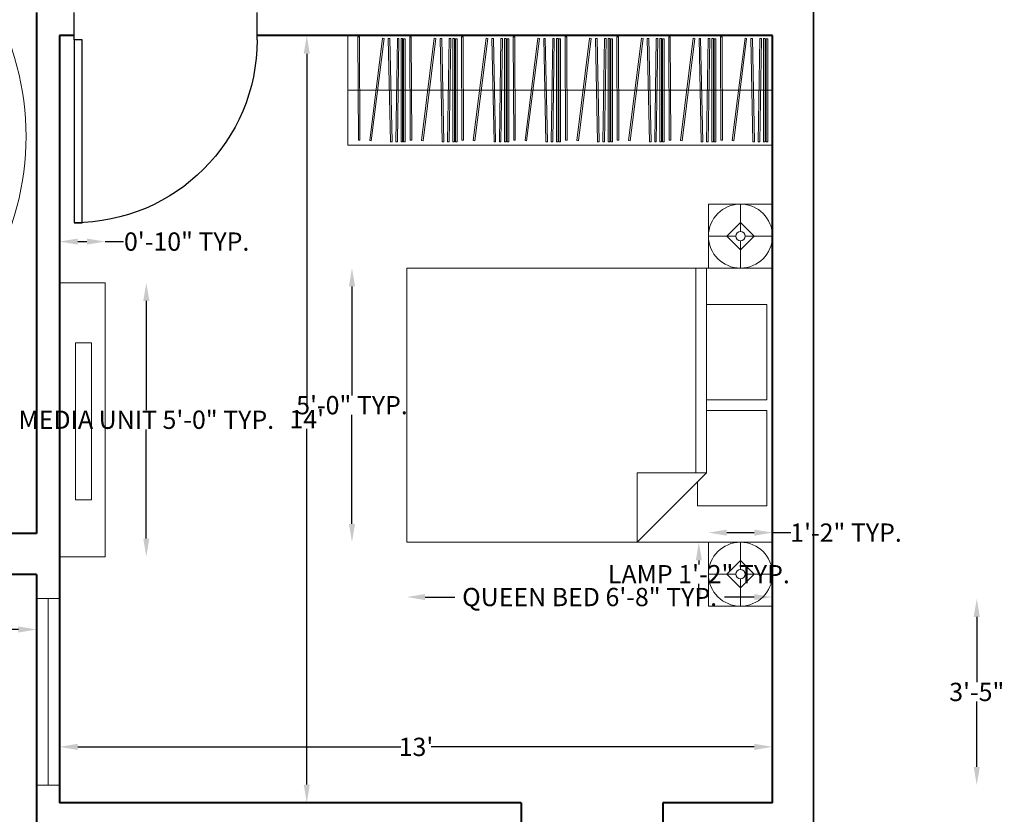
# Model space of a CAD drawing. Units: inches. Extents: x -46 to 447, y -42 to 702.
# Tile 3 of 7: x 222 to 438, y 148 to 322. Entities that reach past the tile are written whole.
import ezdxf

# ---------------------------------------------------------------- set-up
doc = ezdxf.new("R2010")
doc.units = ezdxf.units.IN
doc.header["$PDMODE"] = 3
for name, color, linetype, lineweight in [('A-ANNO-DIMS', 2, 'Continuous', 13), ('A-DOOR', 3, 'Continuous', 25), ('A-FLOR-CASE', 32, 'Continuous', 18), ('A-FURN', 8, 'Continuous', 18), ('A-GLAZ', 4, 'Continuous', 18), ('A-WALL', 7, 'Continuous', 40), ('L-WALL', 7, 'Continuous', 35)]:
    doc.layers.add(name, color=color, linetype=linetype, lineweight=lineweight)
doc.styles.get("Standard").update_dxf_attribs({"font": 'arial.ttf'})
doc.dimstyles.get("Standard").update_dxf_attribs({"dimtxt": 4, "dimasz": 4, "dimexe": 0.18, "dimexo": 0.0625, "dimgap": 0.09, "dimtad": 0, "dimtih": 1, "dimtoh": 1, "dimdec": 0, "dimzin": 0, "dimdsep": 46, "dimlunit": 3, "dimtxsty": 'Standard', "dimcen": 0.09, "dimse1": 1, "dimse2": 1, "dimadec": 0, "dimazin": 0, "dimtfac": 1, "dimtdec": 0, "dimtofl": 0, "dimtmove": 0, "dimatfit": 3, "dimfxl": 1, "dimtolj": 1, "dimtzin": 0, "dimarcsym": 0})

# ---------------------------------------------------------------- blocks, each defined once
blk = doc.blocks.new('*U2')
for p, q in [((0, 0), (0, -6)), ((40, 0), (40, -6))]:
    blk.add_line(p, q)
blk.add_lwpolyline([(0, 0), (0, 40), (1.75, 40), (1.75, 0)], close=True)
blk.add_arc((0, 0), 40, 0, 90)
blk = doc.blocks.new('Sofa - Roundback Loveseat 5 ft.')
for p, q in [((0, -32.44198), (0, -5.99998)), ((-24, -33.99998), (-24, -11.46958)), ((24.00004, -33.99998), (24.00004, -11.46958)), ((-23.9998, -13.38178), (23.99986, -13.38178)), ((-24, -32.44198), (24.00004, -32.44198))]:
    blk.add_line(p, q)
for points in [[(-24, -33.99998), (-30, -33.99998), (-30, -7.99998)], [(30.00004, -7.99998), (30.00004, -33.99998), (24.00004, -33.99998)]]:
    blk.add_lwpolyline(points)
for centre, radius, start, end in [((0, -60.24998), 60.24998, 60.13715, 119.8628), ((0, -61.38438), 55.38444, 64.32083, 115.6792)]:
    blk.add_arc(centre, radius, start, end)
blk = doc.blocks.new('Bed - Queen')
for p, q in [((0, -80.00003), (0, 0)), ((0, 0), (59.99999, 0)), ((59.99999, 0), (59.99999, -80.00003)), ((7.99999, -1.2), (28.79998, -1.2)), ((7.99999, -14.4), (7.99999, -1.2)), ((28.79998, -1.2), (28.79998, -14.4)), ((31.19999, -1.2), (51.99999, -1.2)), ((31.19999, -14.4), (31.19999, -1.2)), ((51.99999, -1.2), (51.99999, -16.4)), ((0, -14.4), (44.8, -14.4)), ((59.99999, -29.6), (44.8, -14.4)), ((44.8, -14.4), (44.8, -29.6)), ((44.8, -16.8), (0, -16.8)), ((51.99999, -16.4), (46.79936, -16.4)), ((44.8, -29.6), (59.99999, -29.6)), ((59.99999, -80.00003), (0, -80.00003))]:
    blk.add_line(p, q)
blk = doc.blocks.new('Lamp - Table')
for p, q in [((0, 7), (0, 1)), ((0, 3), (-3, 0)), ((3, 0), (0, 3)), ((-1, 0), (-7, 0)), ((-3, 0), (0, -3)), ((0, -3), (3, 0)), ((1, 0), (7, 0)), ((0, -1), (0, -7))]:
    blk.add_line(p, q)
for radius in [7, 1]:
    blk.add_circle((0, 0), radius)
blk = doc.blocks.new('*D52')
at = {"layer": 'A-ANNO-DIMS', "color": 0, "lineweight": -2, "transparency": 16777216}
for p, q in [((13, 188.95), (110.73, 188.95)), ((222, 188.95), (124.27, 188.95))]:
    blk.add_line(p, q, dxfattribs=at)
at = {"layer": 'A-ANNO-DIMS', "color": 0, "transparency": 16777216}
for points in [[(13, 189.62), (13, 188.29), (9, 188.95)], [(222, 189.62), (222, 188.29), (226, 188.95)]]:
    blk.add_solid(points, dxfattribs=at)
at = {"layer": 'Defpoints', "color": 0, "transparency": 16777216}
for p in [(226, 188.95), (9, 180.86), (226, 180.86)]:
    blk.add_point(p, dxfattribs=at)
at = {"layer": 'A-ANNO-DIMS', "color": 0, "transparency": 16777216, "insert": (117.5, 188.95), "char_height": 4, "attachment_point": 5}
blk.add_mtext('\\A1;18\'-1"', dxfattribs=at)
blk = doc.blocks.new('*D59')
at = {"layer": 'A-ANNO-DIMS', "color": 0, "lineweight": -2, "transparency": 16777216}
for p, q in [((285.11, 315), (285.11, 237.1)), ((285.11, 155), (285.11, 232.9))]:
    blk.add_line(p, q, dxfattribs=at)
at = {"layer": 'A-ANNO-DIMS', "color": 0, "transparency": 16777216}
for points in [[(284.44, 315), (285.78, 315), (285.11, 319)], [(284.44, 155), (285.78, 155), (285.11, 151)]]:
    blk.add_solid(points, dxfattribs=at)
at = {"layer": 'Defpoints', "color": 0, "transparency": 16777216}
for p in [(285.11, 319), (387, 319), (387, 151)]:
    blk.add_point(p, dxfattribs=at)
at = {"layer": 'A-ANNO-DIMS', "color": 0, "transparency": 16777216, "insert": (285.11, 235), "char_height": 4, "attachment_point": 5}
blk.add_mtext("\\A1;14'", dxfattribs=at)
blk = doc.blocks.new('*D60')
at = {"layer": 'A-ANNO-DIMS', "color": 0, "lineweight": -2, "transparency": 16777216}
for p, q in [((235, 163.26), (305.7, 163.26)), ((383, 163.26), (312.3, 163.26))]:
    blk.add_line(p, q, dxfattribs=at)
at = {"layer": 'A-ANNO-DIMS', "color": 0, "transparency": 16777216}
for points in [[(235, 163.93), (235, 162.59), (231, 163.26)], [(383, 163.93), (383, 162.59), (387, 163.26)]]:
    blk.add_solid(points, dxfattribs=at)
at = {"layer": 'Defpoints', "color": 0, "transparency": 16777216}
for p in [(387, 163.26), (231, 151), (387, 151)]:
    blk.add_point(p, dxfattribs=at)
at = {"layer": 'A-ANNO-DIMS', "color": 0, "transparency": 16777216, "insert": (309, 163.26), "char_height": 4, "attachment_point": 5}
blk.add_mtext("\\A1;13'", dxfattribs=at)
blk = doc.blocks.new('WARDROBE-93X24')
for p, q in [((12, -92.9), (12, 0)), ((24, 0), (24, -92.9)), ((24, -92.9), (0, -92.9))]:
    blk.add_line(p, q)
for points in [[(0.7, -1.6), (23.3, -1.6), (23.3, -1.95), (0.7, -1.95)], [(0.72, -1.03), (23.33, -1.03), (23.33, -1.38), (0.72, -1.38)], [(23.3, -3.1), (0.7, -2.75), (0.7, -2.4), (23.3, -2.75)], [(23.3, -4.26), (0.7, -4.73), (0.7, -4.38), (23.3, -3.91)], [(23.09, -8.46), (0.66, -5.66), (0.61, -6), (23.04, -8.81)], [(22.92, -11.29), (0.31, -11.38), (0.31, -11.03), (22.91, -10.94)], [(0.72, -12.37), (23.33, -12.37), (23.33, -12.72), (0.72, -12.72)], [(0.7, -12.93), (23.3, -12.93), (23.3, -13.28), (0.7, -13.28)], [(23.3, -14.43), (0.7, -14.08), (0.7, -13.73), (23.3, -14.08)], [(23.09, -19.79), (0.66, -16.99), (0.61, -17.34), (23.04, -20.14)], [(23.3, -15.59), (0.7, -16.06), (0.7, -15.71), (23.3, -15.24)], [(22.92, -22.62), (0.31, -22.71), (0.31, -22.36), (22.91, -22.27)], [(0.72, -23.7), (23.33, -23.7), (23.33, -24.05), (0.72, -24.05)], [(0.7, -24.26), (23.3, -24.26), (23.3, -24.61), (0.7, -24.61)], [(23.3, -25.77), (0.7, -25.41), (0.7, -25.06), (23.3, -25.41)], [(23.3, -26.93), (0.7, -27.39), (0.7, -27.04), (23.3, -26.57)], [(23.09, -31.12), (0.66, -28.32), (0.61, -28.67), (23.04, -31.47)], [(22.92, -33.95), (0.31, -34.04), (0.31, -33.69), (22.91, -33.6)], [(0.7, -35.59), (23.3, -35.59), (23.3, -35.94), (0.7, -35.94)], [(23.3, -37.1), (0.7, -36.75), (0.7, -36.39), (23.3, -36.75)], [(0.72, -35.03), (23.33, -35.03), (23.33, -35.38), (0.72, -35.38)], [(23.3, -38.26), (0.7, -38.72), (0.7, -38.37), (23.3, -37.91)], [(23.09, -42.45), (0.66, -39.65), (0.61, -40), (23.04, -42.8)], [(22.92, -45.28), (0.31, -45.37), (0.31, -45.02), (22.91, -44.93)], [(0.7, -46.92), (23.3, -46.92), (23.3, -47.27), (0.7, -47.27)], [(0.72, -46.36), (23.33, -46.36), (23.33, -46.71), (0.72, -46.71)], [(23.3, -48.43), (0.7, -48.08), (0.7, -47.73), (23.3, -48.08)], [(23.3, -49.59), (0.7, -50.05), (0.7, -49.7), (23.3, -49.24)], [(23.09, -53.79), (0.66, -50.98), (0.61, -51.33), (23.04, -54.13)], [(22.92, -56.61), (0.31, -56.7), (0.31, -56.35), (22.91, -56.26)], [(0.72, -57.69), (23.33, -57.69), (23.33, -58.04), (0.72, -58.04)], [(0.7, -58.25), (23.3, -58.25), (23.3, -58.6), (0.7, -58.6)], [(23.3, -59.76), (0.7, -59.41), (0.7, -59.06), (23.3, -59.41)], [(23.09, -65.12), (0.66, -62.31), (0.61, -62.66), (23.04, -65.47)], [(23.3, -60.92), (0.7, -61.39), (0.7, -61.04), (23.3, -60.57)], [(22.92, -67.95), (0.31, -68.04), (0.31, -67.68), (22.91, -67.59)], [(0.7, -69.59), (23.3, -69.59), (23.3, -69.94), (0.7, -69.94)], [(23.3, -71.09), (0.7, -70.74), (0.7, -70.39), (23.3, -70.74)], [(0.72, -69.02), (23.33, -69.02), (23.33, -69.37), (0.72, -69.37)], [(23.3, -72.25), (0.7, -72.72), (0.7, -72.37), (23.3, -71.9)], [(23.09, -76.45), (0.66, -73.64), (0.61, -73.99), (23.04, -76.8)], [(22.92, -79.28), (0.31, -79.37), (0.31, -79.02), (22.91, -78.93)], [(0.7, -80.92), (23.3, -80.92), (23.3, -81.27), (0.7, -81.27)], [(23.3, -82.42), (0.7, -82.07), (0.7, -81.72), (23.3, -82.07)], [(0.72, -80.35), (23.33, -80.35), (23.33, -80.71), (0.72, -80.71)], [(23.3, -83.58), (0.7, -84.05), (0.7, -83.7), (23.3, -83.23)], [(23.09, -87.78), (0.66, -84.98), (0.61, -85.32), (23.04, -88.13)], [(22.92, -90.61), (0.31, -90.7), (0.31, -90.35), (22.91, -90.26)]]:
    blk.add_lwpolyline(points, close=True)
blk = doc.blocks.new('MEDIA-CONSOLE-60')
for points in [[(60, 0), (0, 0), (0, 10), (60, 10)], [(13.13, 6.99), (47.53, 6.99), (47.53, 3.54), (13.13, 3.54)]]:
    blk.add_lwpolyline(points, close=True)
blk = doc.blocks.new('NIGHTSTAND-14')
blk.add_lwpolyline([(0, 0), (0, -14.000002), (14.000002, -14.000002), (14.000002, 0)], close=True)
blk = doc.blocks.new('*D84')
at = {"layer": 'A-ANNO-DIMS', "color": 0, "lineweight": -2, "transparency": 16777216}
for p, q in [((311, 196.06), (317.49, 196.06)), ((383, 196.06), (376.51, 196.06))]:
    blk.add_line(p, q, dxfattribs=at)
at = {"layer": 'A-ANNO-DIMS', "color": 0, "transparency": 16777216}
for points in [[(311, 196.72), (311, 195.39), (307, 196.06)], [(383, 196.72), (383, 195.39), (387, 196.06)]]:
    blk.add_solid(points, dxfattribs=at)
at = {"layer": 'Defpoints', "color": 0, "transparency": 16777216}
for p in [(307, 208.06), (387, 208.06), (387, 196.06)]:
    blk.add_point(p, dxfattribs=at)
at = {"layer": 'A-ANNO-DIMS', "color": 0, "transparency": 16777216, "insert": (347, 196.06), "char_height": 4, "attachment_point": 5}
blk.add_mtext('\\A1;QUEEN BED 6\'-8" TYP.', dxfattribs=at)
blk = doc.blocks.new('*D85')
at = {"layer": 'A-ANNO-DIMS', "color": 0, "lineweight": -2, "transparency": 16777216}
for p, q in [((295, 264.06), (295, 240.19)), ((295, 212.06), (295, 235.92))]:
    blk.add_line(p, q, dxfattribs=at)
at = {"layer": 'A-ANNO-DIMS', "color": 0, "transparency": 16777216}
for points in [[(294.33, 264.06), (295.67, 264.06), (295, 268.06)], [(294.33, 212.06), (295.67, 212.06), (295, 208.06)]]:
    blk.add_solid(points, dxfattribs=at)
at = {"layer": 'Defpoints', "color": 0, "transparency": 16777216}
for p in [(307, 268.06), (295, 208.06), (307, 208.06)]:
    blk.add_point(p, dxfattribs=at)
at = {"layer": 'A-ANNO-DIMS', "color": 0, "transparency": 16777216, "insert": (295, 238.06), "char_height": 4, "attachment_point": 5}
blk.add_mtext('\\A1;5\'-0" TYP.', dxfattribs=at)
blk = doc.blocks.new('*D88')
at = {"layer": 'A-ANNO-DIMS', "color": 0, "lineweight": -2, "transparency": 16777216}
for p, q in [((250, 260.87), (250, 237)), ((250, 208.87), (250, 232.74))]:
    blk.add_line(p, q, dxfattribs=at)
at = {"layer": 'A-ANNO-DIMS', "color": 0, "transparency": 16777216}
for points in [[(249.33, 260.87), (250.67, 260.87), (250, 264.87)], [(249.33, 208.87), (250.67, 208.87), (250, 204.87)]]:
    blk.add_solid(points, dxfattribs=at)
at = {"layer": 'Defpoints', "color": 0, "transparency": 16777216}
for p in [(241, 264.87), (241, 204.87), (250, 204.87)]:
    blk.add_point(p, dxfattribs=at)
at = {"layer": 'A-ANNO-DIMS', "color": 0, "transparency": 16777216, "insert": (250, 234.87), "char_height": 4, "attachment_point": 5}
blk.add_mtext('\\A1;MEDIA UNIT 5\'-0" TYP.', dxfattribs=at)
blk = doc.blocks.new('*D89')
at = {"layer": 'A-ANNO-DIMS', "color": 0, "lineweight": -2, "transparency": 16777216}
for p, q in [((235, 273.87), (237, 273.87)), ((241, 273.87), (245, 273.87))]:
    blk.add_line(p, q, dxfattribs=at)
at = {"layer": 'A-ANNO-DIMS', "color": 0, "transparency": 16777216}
for points in [[(235, 274.53), (235, 273.2), (231, 273.87)], [(237, 274.53), (237, 273.2), (241, 273.87)]]:
    blk.add_solid(points, dxfattribs=at)
at = {"layer": 'Defpoints', "color": 0, "transparency": 16777216}
for p in [(241, 273.87), (231, 264.87), (241, 264.87)]:
    blk.add_point(p, dxfattribs=at)
at = {"layer": 'A-ANNO-DIMS', "color": 0, "transparency": 16777216, "insert": (258.83, 273.87), "char_height": 4, "attachment_point": 5}
blk.add_mtext('\\A1;0\'-10" TYP.', dxfattribs=at)
blk = doc.blocks.new('*D92')
at = {"layer": 'A-ANNO-DIMS', "color": 0, "lineweight": -2, "transparency": 16777216}
for p, q in [((370.9, 204.06), (370.9, 203.16)), ((370.9, 198.06), (370.9, 198.96))]:
    blk.add_line(p, q, dxfattribs=at)
at = {"layer": 'A-ANNO-DIMS', "color": 0, "transparency": 16777216}
for points in [[(370.23, 204.06), (371.57, 204.06), (370.9, 208.06)], [(370.23, 198.06), (371.57, 198.06), (370.9, 194.06)]]:
    blk.add_solid(points, dxfattribs=at)
at = {"layer": 'Defpoints', "color": 0, "transparency": 16777216}
for p in [(370.9, 208.06), (373, 208.06), (373, 194.06)]:
    blk.add_point(p, dxfattribs=at)
at = {"layer": 'A-ANNO-DIMS', "color": 0, "transparency": 16777216, "insert": (370.9, 201.06), "char_height": 4, "attachment_point": 5}
blk.add_mtext('\\A1;LAMP 1\'-2" TYP.', dxfattribs=at)
blk = doc.blocks.new('*D93')
at = {"layer": 'A-ANNO-DIMS', "color": 0, "lineweight": -2, "transparency": 16777216}
for p, q in [((377, 210.16), (383, 210.16)), ((387, 210.16), (391, 210.16))]:
    blk.add_line(p, q, dxfattribs=at)
at = {"layer": 'A-ANNO-DIMS', "color": 0, "transparency": 16777216}
for points in [[(377, 210.82), (377, 209.49), (373, 210.16)], [(383, 210.82), (383, 209.49), (387, 210.16)]]:
    blk.add_solid(points, dxfattribs=at)
at = {"layer": 'Defpoints', "color": 0, "transparency": 16777216}
for p in [(387, 210.16), (373, 208.06), (387, 208.06)]:
    blk.add_point(p, dxfattribs=at)
at = {"layer": 'A-ANNO-DIMS', "color": 0, "transparency": 16777216, "insert": (403.09, 210.16), "char_height": 4, "attachment_point": 5}
blk.add_mtext('\\A1;1\'-2" TYP.', dxfattribs=at)
blk = doc.blocks.new('*D118')
at = {"layer": 'A-ANNO-DIMS', "color": 0, "lineweight": -2, "transparency": 16777216}
for p, q in [((352, -35.7), (362.09, -35.7)), ((383, -35.7), (372.91, -35.7))]:
    blk.add_line(p, q, dxfattribs=at)
at = {"layer": 'A-ANNO-DIMS', "color": 0, "transparency": 16777216}
for points in [[(352, -35.03), (352, -36.37), (348, -35.7)], [(383, -35.03), (383, -36.37), (387, -35.7)]]:
    blk.add_solid(points, dxfattribs=at)
at = {"layer": 'Defpoints', "color": 0, "transparency": 16777216}
for p in [(348, 324), (387, 324), (387, -35.7)]:
    blk.add_point(p, dxfattribs=at)
at = {"layer": 'A-ANNO-DIMS', "color": 0, "transparency": 16777216, "insert": (367.5, -35.7), "char_height": 4, "attachment_point": 5}
blk.add_mtext('\\A1;3\'-3"', dxfattribs=at)
blk = doc.blocks.new('*D119')
at = {"layer": 'A-ANNO-DIMS', "color": 0, "lineweight": -2, "transparency": 16777216}
for p, q in [((238.24, 695.7), (248.83, 695.7)), ((270.24, 695.7), (259.64, 695.7))]:
    blk.add_line(p, q, dxfattribs=at)
at = {"layer": 'A-ANNO-DIMS', "color": 0, "transparency": 16777216}
for points in [[(238.24, 696.37), (238.24, 695.03), (234.24, 695.7)], [(270.24, 696.37), (270.24, 695.03), (274.24, 695.7)]]:
    blk.add_solid(points, dxfattribs=at)
at = {"layer": 'Defpoints', "color": 0, "transparency": 16777216}
for p in [(274.24, 695.7), (234.24, 319), (274.24, 319)]:
    blk.add_point(p, dxfattribs=at)
at = {"layer": 'A-ANNO-DIMS', "color": 0, "transparency": 16777216, "insert": (254.24, 695.7), "char_height": 4, "attachment_point": 5}
blk.add_mtext('\\A1;3\'-4"', dxfattribs=at)
blk = doc.blocks.new('*D120')
at = {"layer": 'A-ANNO-DIMS', "color": 0, "lineweight": -2, "transparency": 16777216}
for p, q in [((336, -35.7), (342.06, -35.7)), ((359, -35.7), (352.94, -35.7))]:
    blk.add_line(p, q, dxfattribs=at)
at = {"layer": 'A-ANNO-DIMS', "color": 0, "transparency": 16777216}
for points in [[(336, -35.03), (336, -36.37), (332, -35.7)], [(359, -35.03), (359, -36.37), (363, -35.7)]]:
    blk.add_solid(points, dxfattribs=at)
at = {"layer": 'Defpoints', "color": 0, "transparency": 16777216}
for p in [(332, 151), (363, 151), (363, -35.7)]:
    blk.add_point(p, dxfattribs=at)
at = {"layer": 'A-ANNO-DIMS', "color": 0, "transparency": 16777216, "insert": (347.5, -35.7), "char_height": 4, "attachment_point": 5}
blk.add_mtext('\\A1;2\'-7"', dxfattribs=at)
blk = doc.blocks.new('*D133')
at = {"layer": 'A-ANNO-DIMS', "color": 0, "lineweight": -2, "transparency": 16777216}
for p, q in [((431.7, 191.71), (431.7, 177.43)), ((431.7, 158.88), (431.7, 173.16))]:
    blk.add_line(p, q, dxfattribs=at)
at = {"layer": 'A-ANNO-DIMS', "color": 0, "transparency": 16777216}
for points in [[(431.03, 191.71), (432.37, 191.71), (431.7, 195.71)], [(431.03, 158.88), (432.37, 158.88), (431.7, 154.88)]]:
    blk.add_solid(points, dxfattribs=at)
at = {"layer": 'Defpoints', "color": 0, "transparency": 16777216}
for p in [(231, 195.71), (431.7, 195.71), (231, 154.88)]:
    blk.add_point(p, dxfattribs=at)
at = {"layer": 'A-ANNO-DIMS', "color": 0, "transparency": 16777216, "insert": (431.7, 175.29), "char_height": 4, "attachment_point": 5}
blk.add_mtext('\\A1;3\'-5"', dxfattribs=at)
blk = doc.blocks.new('*D143')
at = {"layer": 'A-ANNO-DIMS', "color": 0, "lineweight": -2, "transparency": 16777216}
for p, q in [((220.17, -35.7), (222, -35.7)), ((226, -35.7), (230, -35.7))]:
    blk.add_line(p, q, dxfattribs=at)
at = {"layer": 'A-ANNO-DIMS', "color": 0, "transparency": 16777216}
for points in [[(220.17, -35.03), (220.17, -36.37), (216.17, -35.7)], [(222, -35.03), (222, -36.37), (226, -35.7)]]:
    blk.add_solid(points, dxfattribs=at)
at = {"layer": 'Defpoints', "color": 0, "transparency": 16777216}
for p in [(216.17, 201), (226, 201), (226, -35.7)]:
    blk.add_point(p, dxfattribs=at)
at = {"layer": 'A-ANNO-DIMS', "color": 0, "transparency": 16777216, "insert": (236.96, -35.7), "char_height": 4, "attachment_point": 5}
blk.add_mtext('\\A1;0\'-10"', dxfattribs=at)
blk = doc.blocks.new('*D147')
at = {"layer": 'A-ANNO-DIMS', "color": 0, "lineweight": -2, "transparency": 16777216}
for p, q in [((367, -35.7), (369.56, -35.7)), ((383, -35.7), (380.44, -35.7))]:
    blk.add_line(p, q, dxfattribs=at)
at = {"layer": 'A-ANNO-DIMS', "color": 0, "transparency": 16777216}
for points in [[(367, -35.03), (367, -36.37), (363, -35.7)], [(383, -35.03), (383, -36.37), (387, -35.7)]]:
    blk.add_solid(points, dxfattribs=at)
at = {"layer": 'Defpoints', "color": 0, "transparency": 16777216}
for p in [(363, 151), (387, 151), (387, -35.7)]:
    blk.add_point(p, dxfattribs=at)
at = {"layer": 'A-ANNO-DIMS', "color": 0, "transparency": 16777216, "insert": (375, -35.7), "char_height": 4, "attachment_point": 5}
blk.add_mtext('\\A1;2\'-0"', dxfattribs=at)
blk = doc.blocks.new('*D148')
at = {"layer": 'A-ANNO-DIMS', "color": 0, "lineweight": -2, "transparency": 16777216}
for p, q in [((227, 695.7), (223, 695.7)), ((238.24, 695.7), (242.24, 695.7))]:
    blk.add_line(p, q, dxfattribs=at)
at = {"layer": 'A-ANNO-DIMS', "color": 0, "transparency": 16777216}
for points in [[(227, 696.37), (227, 695.03), (231, 695.7)], [(238.24, 696.37), (238.24, 695.03), (234.24, 695.7)]]:
    blk.add_solid(points, dxfattribs=at)
at = {"layer": 'Defpoints', "color": 0, "transparency": 16777216}
for p in [(234.24, 695.7), (231, 319), (234.24, 319)]:
    blk.add_point(p, dxfattribs=at)
at = {"layer": 'A-ANNO-DIMS', "color": 0, "transparency": 16777216, "insert": (247.64, 695.7), "char_height": 4, "attachment_point": 5}
blk.add_mtext('\\A1;0\'-3"', dxfattribs=at)

msp = doc.modelspace()

# ---------------------------------------------------------------- linework, layer by layer
at = {"layer": 'A-FLOR-CASE'}
for p in [(294.1, 319), (387, 295)]:
    msp.add_line(p, (387, 319), dxfattribs=at)
at = {"layer": 'A-GLAZ'}
for p, q in [((226, 195.71), (231, 195.71)), ((228.5, 195.71), (228.5, 154.88)), ((226, 154.88), (231, 154.88))]:
    msp.add_line(p, q, dxfattribs=at)
at = {"layer": 'A-WALL'}
for p, q in [((226, 324), (226, 210)), ((231, 319), (231, 151)), ((234.24, 319), (231, 319)), ((387, 319), (274.24, 319)), ((387, 151), (387, 319)), ((226, 210), (214.42, 210)), ((226, 201), (216.17, 201)), ((226, 201), (226, 84)), ((332, 151), (231, 151)), ((332, 151), (332, 145.1)), ((387, 151), (363, 151)), ((363, 151), (363, 146))]:
    msp.add_line(p, q, dxfattribs=at)
at = {"layer": 'L-WALL'}
msp.add_lwpolyline([(222, 0), (396, 0), (396, 660), (0, 660), (0, 0), (17.93, 0)], dxfattribs=at)

# ---------------------------------------------------------------- block references
at = {"layer": 'A-DOOR', "xscale": -1, "rotation": 180}
msp.add_blockref('*U2', (234.24, 318), dxfattribs=at)
at = {"layer": 'A-FLOR-CASE'}
for name, p, rotation in [('WARDROBE-93X24', (387, 319), 270.0000000000001), ('MEDIA-CONSOLE-60', (231, 264.87), 269.9999999999999)]:
    msp.add_blockref(name, p, dxfattribs=dict(at, rotation=rotation))
at = {"layer": 'A-FURN', "xscale": -1, "rotation": 270}
for name, p in [('Sofa - Roundback Loveseat 5 ft.', (223.68, 296.9)), ('Lamp - Table', (380, 201.06))]:
    msp.add_blockref(name, p, dxfattribs=at)
at = {"layer": 'A-FURN'}
for name, p, rotation in [('Lamp - Table', (380, 275.06), 270), ('NIGHTSTAND-14', (387, 282.06), 270.0000000000002), ('Bed - Queen', (387, 268.06), 270), ('NIGHTSTAND-14', (387, 194.06), 180)]:
    msp.add_blockref(name, p, dxfattribs=dict(at, rotation=rotation))

# ---------------------------------------------------------------- dimensions: what is measured, and where the dimension line sits
at = {"layer": 'A-ANNO-DIMS'}
for base, p1, p2, override, picture, middle in [((234.24, 695.7), (231, 319), (234.24, 319), {"dimdec": 1, "dimlfac": 1, "dimrnd": 0, "dimzin": 1, "dimdsep": 46, "dimlunit": 4, "dimfrac": 2}, '*D148', (247.64, 695.7)), ((274.24, 695.7), (234.24, 319), (274.24, 319), {"dimdec": 1, "dimlfac": 1, "dimrnd": 0, "dimzin": 1, "dimdsep": 46, "dimlunit": 4, "dimfrac": 2}, '*D119', (254.24, 695.7)), ((387, -35.7), (348, 324), (387, 324), {"dimdec": 1, "dimlfac": 1, "dimrnd": 0, "dimzin": 1, "dimdsep": 46, "dimlunit": 4, "dimfrac": 2}, '*D118', (367.5, -35.7)), ((226, -35.7), (216.17, 201), (226, 201), {"dimdec": 1, "dimlfac": 1, "dimrnd": 0, "dimzin": 1, "dimdsep": 46, "dimlunit": 4, "dimfrac": 2}, '*D143', (236.96, -35.7)), ((226, 188.95), (9, 180.86), (226, 180.86), {"dimclrd": 0, "dimclre": 0, "dimclrt": 0}, '*D52', (117.5, 188.95)), ((387, 163.26), (231, 151), (387, 151), {"dimclrd": 0, "dimclre": 0, "dimclrt": 0}, '*D60', (309, 163.26)), ((363, -35.7), (332, 151), (363, 151), {"dimdec": 1, "dimlfac": 1, "dimrnd": 0, "dimzin": 1, "dimdsep": 46, "dimlunit": 4, "dimfrac": 2}, '*D120', (347.5, -35.7)), ((387, -35.7), (363, 151), (387, 151), {"dimdec": 1, "dimlfac": 1, "dimrnd": 0, "dimzin": 1, "dimdsep": 46, "dimlunit": 4, "dimfrac": 2}, '*D147', (375, -35.7))]:
    dim = msp.add_linear_dim(base=base, p1=p1, p2=p2, dimstyle='Standard', override=override, dxfattribs=at)
    dim.commit()
    dim.dimension.update_dxf_attribs({"geometry": picture, "text_midpoint": middle})
for base, p1, p2, override, picture, middle in [((285.11, 319), (387, 151), (387, 319), {"dimclrd": 0, "dimclre": 0, "dimclrt": 0}, '*D59', (285.11, 235)), ((431.7, 195.71), (231, 154.88), (231, 195.71), {"dimdec": 1, "dimlfac": 1, "dimrnd": 0, "dimzin": 1, "dimdsep": 46, "dimlunit": 4, "dimfrac": 2}, '*D133', (431.7, 175.29))]:
    dim = msp.add_linear_dim(base=base, p1=p1, p2=p2, angle=90, dimstyle='Standard', override=override, dxfattribs=at)
    dim.commit()
    dim.dimension.update_dxf_attribs({"geometry": picture, "text_midpoint": middle})
for base, p1, p2, text, picture, middle in [((241, 273.87), (231, 264.87), (241, 264.87), '<> TYP.', '*D89', (258.83, 273.87)), ((387, 210.16), (373, 208.06), (387, 208.06), '<> TYP.', '*D93', (403.09, 210.16)), ((387, 196.06), (307, 208.06), (387, 208.06), 'QUEEN BED <> TYP.', '*D84', (347, 196.06))]:
    dim = msp.add_linear_dim(base=base, p1=p1, p2=p2, text=text, dimstyle='Standard', override={"dimdec": 1, "dimlfac": 1, "dimrnd": 0, "dimzin": 1, "dimdsep": 46, "dimlunit": 4, "dimfrac": 2}, dxfattribs=at)
    dim.commit()
    dim.dimension.update_dxf_attribs({"geometry": picture, "text_midpoint": middle})
for base, p1, p2, angle, text, picture, middle in [((295, 208.06), (307, 268.06), (307, 208.06), 270, '<> TYP.', '*D85', (295, 238.06)), ((250, 204.87), (241, 264.87), (241, 204.87), 270, 'MEDIA UNIT <> TYP.', '*D88', (250, 234.87)), ((370.9, 208.06), (373, 194.06), (373, 208.06), 90, 'LAMP <> TYP.', '*D92', (370.9, 201.06))]:
    dim = msp.add_linear_dim(base=base, p1=p1, p2=p2, angle=angle, text=text, dimstyle='Standard', override={"dimdec": 1, "dimlfac": 1, "dimrnd": 0, "dimzin": 1, "dimdsep": 46, "dimlunit": 4, "dimfrac": 2}, dxfattribs=at)
    dim.commit()
    dim.dimension.update_dxf_attribs({"geometry": picture, "text_midpoint": middle})

doc.saveas('drawing.dxf')
